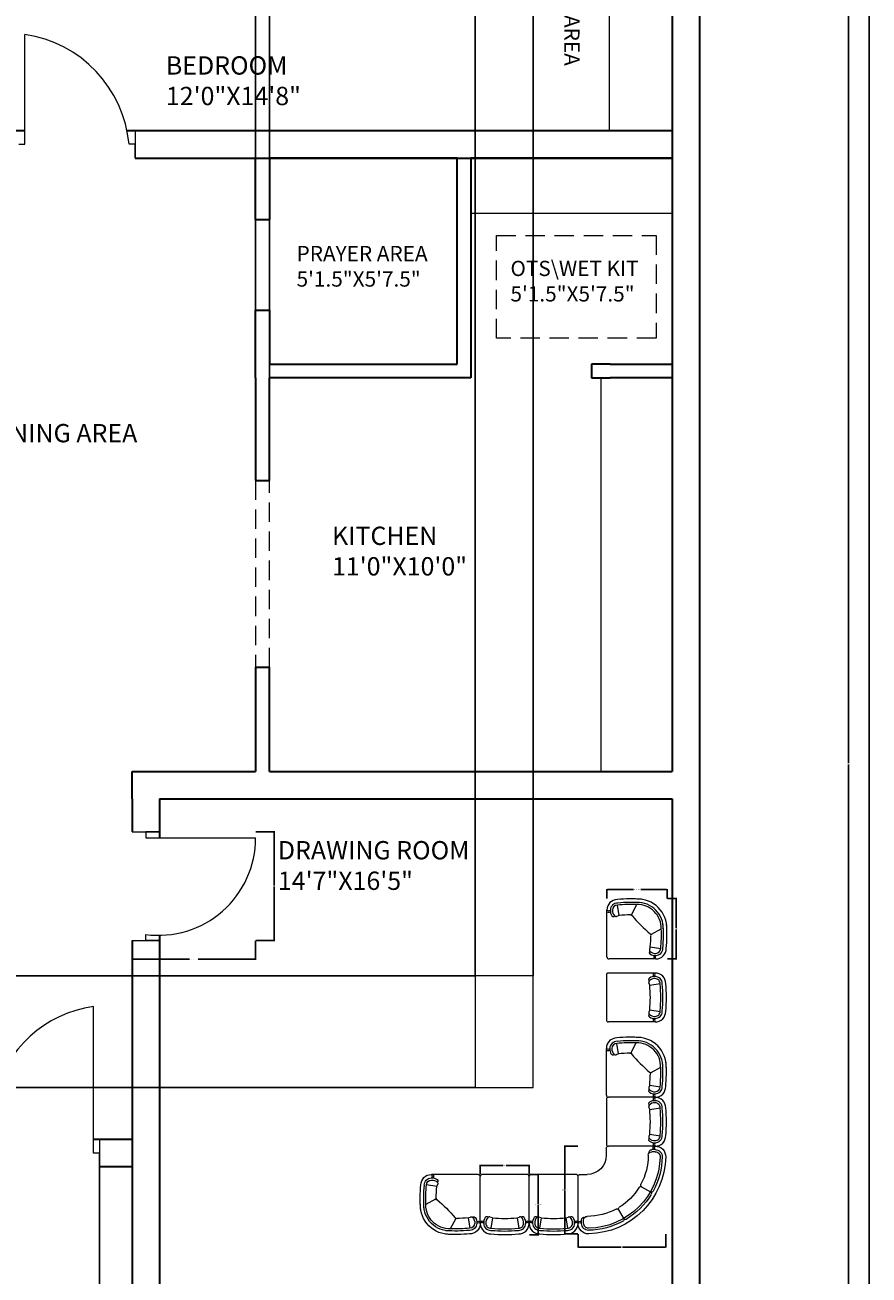
# Model space of a CAD drawing. Units: inches. Extents: x 2460 to 3031, y 933 to 2010.
# Tile 6 of 7: x 2754 to 3031, y 1339 to 1749. Entities that reach past the tile are written whole.
import ezdxf

# ---------------------------------------------------------------- set-up
doc = ezdxf.new("R2010")
doc.units = ezdxf.units.IN
doc.linetypes.add('DASHED2', pattern=[9.525, 6.35, -3.175])
for name, color, linetype, lineweight in [('A-ANNO-DIMS', 2, 'Continuous', 18), ('A-ANNO-TTLB', 7, 'Continuous', 25), ('A-AREA-IDEN', 7, 'Continuous', 18), ('A-DOOR', 4, 'Continuous', 18), ('A-FLOR-CASE', 9, 'Continuous', 18), ('A-FLOR-OVHD', 254, 'DASHED2', 13), ('A-FURN', 8, 'Continuous', 18), ('A-WALL', 7, 'Continuous', 35), ('A-WALL-OVHD', 254, 'DASHED2', 13), ('C-PROP', 7, 'Continuous', 35)]:
    doc.layers.add(name, color=color, linetype=linetype, lineweight=lineweight)
doc.styles.get("Standard").update_dxf_attribs({"font": 'arial.ttf'})
doc.dimstyles.get("Standard").update_dxf_attribs({"dimtxt": 0.18, "dimasz": 0.18, "dimexe": 0.18, "dimexo": 0.0625, "dimgap": 0.09, "dimtad": 0, "dimtih": 1, "dimtoh": 1, "dimdec": 4, "dimzin": 0, "dimdsep": 46, "dimtxsty": 'Standard', "dimcen": 0.09, "dimadec": 0, "dimazin": 0, "dimtfac": 1, "dimtdec": 4, "dimtofl": 0, "dimtmove": 0, "dimatfit": 3, "dimfxl": 1, "dimtolj": 1, "dimtzin": 0, "dimarcsym": 0})

# ---------------------------------------------------------------- blocks, each defined once
blk = doc.blocks.new('A$C707258B2')
at = {"color": 0}
for p, q in [((0.404, 0.342), (1.074, 0.342)), ((0.404, 0.292), (0.454, 0.292)), ((0.404, 0.262), (0.454, 0.262)), ((1.104, 0.312), (1.104, 0.212)), ((1.479, -0.063), (1.379, -0.063)), ((1.509, -0.763), (1.509, -0.093)), ((0.6, -0.238), (0.47, -0.313)), ((0.929, -0.567), (0.854, -0.697)), ((1.429, -0.763), (1.429, -0.713)), ((1.459, -0.763), (1.459, -0.712))]:
    blk.add_line(p, q, dxfattribs=at)
for centre, radius, start, end in [((0.404, 0.192), 0.15, 90, 181.1754), ((1.379, 0.212), 1.125, 181.1754, 268.8246), ((0.404, 0.192), 0.1, 90, 181.1754), ((1.379, 0.212), 1.075, 181.1754, 208.6357), ((0.404, 0.192), 0.07, 90, 181.1754), ((1.379, 0.212), 1.045, 181.1754, 268.8246), ((0.378, 0.317), 0.0362, 316.3972, 43.6028), ((0.368, 0.317), 0.0662, 337.8298, 22.1702), ((0.455, 0.256), 0.0357, 345.4262, 90.5555), ((0.454, 0.212), 0.05, 360, 90), ((1.379, 0.212), 0.875, 180, 208.4082), ((1.074, 0.312), 0.03, 360, 90), ((1.379, 0.212), 0.275, 180, 270), ((1.479, -0.093), 0.03, 360, 90), ((0.457, -0.291), 0.025, 208.6357, 300), ((0.482, -0.334), 0.025, 120, 211.3643), ((1.379, 0.212), 1.075, 211.3643, 238.6357), ((0.587, -0.216), 0.025, 300, 28.4082), ((0.612, -0.259), 0.025, 31.5918, 120), ((1.379, 0.212), 0.875, 211.5918, 238.4082), ((0.907, -0.555), 0.025, 330, 58.4082), ((0.832, -0.685), 0.025, 238.6357, 330), ((0.876, -0.71), 0.025, 150, 241.3643), ((0.951, -0.58), 0.025, 61.5918, 150), ((1.379, 0.212), 0.875, 241.5918, 270), ((1.379, -0.713), 0.05, 360, 90), ((1.425, -0.709), 0.0336, 354.6301, 109.3883), ((1.379, 0.212), 1.075, 241.3643, 268.8246), ((1.359, -0.763), 0.15, 268.8246, 360), ((1.359, -0.763), 0.1, 268.8246, 360), ((1.359, -0.763), 0.07, 268.8246, 360), ((1.484, -0.799), 0.0662, 67.8298, 112.1702), ((1.484, -0.789), 0.0362, 46.3972, 133.6028)]:
    blk.add_arc(centre, radius, start, end, dxfattribs=at)
blk = doc.blocks.new('part 01')
at = {"color": 0}
for p, q in [((-591, 527), (-740, 550)), ((-670, 700), (0, 700)), ((-591, 527), (-579, 561)), ((30, 30), (30, 670)), ((-591, 173), (-740, 150)), ((-670, 0), (0, 0)), ((-591, 173), (-579, 139))]:
    blk.add_line(p, q, dxfattribs=at)
for centre, radius, start, end in [((1178, 350), 2008, 174.2835, 185.7165), ((-670, 550), 150, 90, 181.1754), ((1178, 350), 1958, 174.2835, 185.7165), ((-670, 550), 100, 90, 181.1754), ((1178, 350), 1928, 174.2835, 185.7165), ((-670, 550), 70, 90, 181.1754), ((-660, 518), 133, 56.0897, 95.6132), ((-696, 675), 36.2, 316.3972, 43.6028), ((-660, 518), 103, 42.0066, 95.6132), ((-706, 675), 66.2, 337.8298, 22.1702), ((-600, 607), 25, 332.9608, 56.0897), ((-625, 620), 53.2, 321.0017, 332.9608), ((-602, 570), 25, 340, 42.0066), ((0, 670), 30, 0, 90), ((1178, 350), 1778, 174.2835, 185.7165), ((-670, 150), 150, 178.8246, 270), ((-670, 150), 100, 178.8246, 270), ((-670, 150), 70, 178.8246, 270), ((-660, 182), 133, 264.3868, 303.9103), ((-660, 182), 103, 264.3868, 317.9934), ((-696, 25), 36.2, 316.3972, 43.6028), ((-706, 25), 66.2, 337.8298, 22.1702), ((-600, 93), 25, 303.9103, 27.0392), ((-602, 130), 25, 317.9934, 20), ((-625, 80), 53.2, 27.0392, 38.9983), ((0, 30), 30, 270, 0)]:
    blk.add_arc(centre, radius, start, end, dxfattribs=at)
blk = doc.blocks.new('part02')
at = {"color": 0}
for p, q in [((0, -670), (0, 0)), ((30, 30), (700, 30)), ((621, -143), (609, -109)), ((621, -143), (770, -120)), ((640, -326), (778, -399)), ((173, -591), (139, -579)), ((173, -591), (150, -740)), ((356, -610), (429, -748))]:
    blk.add_line(p, q, dxfattribs=at)
for centre, radius, start, end in [((30, 0), 30, 90, 180), ((726, 5), 56.2, 153.6122, 206.6666), ((726, 5), 36.2, 136.3972, 223.6028), ((700, -120), 150, 0, 90), ((630, -63), 25, 123.9103, 207.0392), ((655, -50), 53.2, 207.0392, 218.9983), ((632, -100), 25, 137.9934, 200), ((690, -152), 103, 84.3868, 137.9934), ((689, -151), 132, 85.4378, 123.9887), ((-1148, -320), 1778, 0.3836, 5.7165), ((700, -121), 101, 357.5006, 89.858), ((700, -120), 70, 0, 90), ((-1228, -320), 2008, 357.7349, 5.7032), ((-1148, -320), 1958, 355.8657, 5.7165), ((-1148, -320), 2008, 355.818, 5.7165), ((2220, -2190), 2454, 130.6961, 139.3039), ((632, -344), 20, 62, 130.6961), ((650, -308), 20, 180.3836, 242), ((439, -409), 419, 268.2181, 1.7819), ((439, -409), 369, 268.2181, 1.7819), ((439, -409), 339, 268.2181, 1.7819), ((25, -696), 56.2, 63.3334, 116.3878), ((25, -696), 36.2, 46.3972, 133.6028), ((150, -670), 150, 180, 271.1754), ((182, -660), 133, 146.0897, 185.6132), ((150, -670), 100, 180, 271.1754), ((93, -600), 25, 62.9608, 146.0897), ((182, -660), 103, 132.0066, 185.6132), ((150, -670), 70, 180, 270), ((80, -625), 53.2, 51.0017, 62.9608), ((130, -602), 25, 70, 132.0066), ((350, 1178), 1778, 264.2835, 269.6164), ((338, -620), 20, 28, 89.6164), ((374, -602), 20, 139.3039, 208), ((350, 1258), 2008, 264.2968, 272.2651), ((350, 1178), 2008, 264.2835, 274.182), ((350, 1178), 1958, 264.2835, 274.1343)]:
    blk.add_arc(centre, radius, start, end, dxfattribs=at)
blk = doc.blocks.new('DOOR-SWING-36')
for p, q in [((0, 35.65), (9, 35.65)), ((4.5, 35.65), (4.5, 33.65)), ((4.5, 33.65), (40.5, 33.65)), ((4.5, 0), (4.5, 2)), ((0, 0), (9, 0)), ((9, 0), (4.5, 0))]:
    blk.add_line(p, q)
blk.add_arc((8.58, 33.65), 31.92, 262.6481, 0)
blk = doc.blocks.new('*D18')
at = {"layer": 'A-ANNO-DIMS', "color": 0, "lineweight": -2, "transparency": 16777216}
for p, q in [((2919.36, 1372.43), (2922.44, 1372.43)), ((2922.26, 1372.25), (2922.26, 1362.73)), ((2922.26, 1352.85), (2922.26, 1362.37)), ((2919.36, 1352.67), (2922.44, 1352.67))]:
    blk.add_line(p, q, dxfattribs=at)
at = {"layer": 'A-ANNO-DIMS', "color": 0, "transparency": 16777216}
for points in [[(2922.23, 1372.25), (2922.29, 1372.25), (2922.26, 1372.43)], [(2922.23, 1352.85), (2922.29, 1352.85), (2922.26, 1352.67)]]:
    blk.add_solid(points, dxfattribs=at)
at = {"layer": 'Defpoints', "color": 0, "transparency": 16777216}
for p in [(2919.29, 1372.43), (2922.26, 1372.43), (2919.29, 1352.67)]:
    blk.add_point(p, dxfattribs=at)
at = {"layer": 'A-ANNO-DIMS', "color": 0, "transparency": 16777216, "insert": (2922.26, 1362.55), "char_height": 0.18, "attachment_point": 5}
blk.add_mtext('\\A1;SOFA SEAT 20 TYP.', dxfattribs=at)
blk = doc.blocks.new('*D19')
at = {"layer": 'A-ANNO-DIMS', "color": 0, "lineweight": -2, "transparency": 16777216}
for p, q in [((2903.27, 1372.49), (2903.27, 1375.57)), ((2903.45, 1375.39), (2910.76, 1375.39)), ((2919.11, 1375.39), (2911.8, 1375.39)), ((2919.29, 1372.49), (2919.29, 1375.57))]:
    blk.add_line(p, q, dxfattribs=at)
at = {"layer": 'A-ANNO-DIMS', "color": 0, "transparency": 16777216}
for points in [[(2903.45, 1375.42), (2903.45, 1375.36), (2903.27, 1375.39)], [(2919.11, 1375.42), (2919.11, 1375.36), (2919.29, 1375.39)]]:
    blk.add_solid(points, dxfattribs=at)
at = {"layer": 'Defpoints', "color": 0, "transparency": 16777216}
for p in [(2903.27, 1375.39), (2903.27, 1372.43), (2919.29, 1372.43)]:
    blk.add_point(p, dxfattribs=at)
at = {"layer": 'A-ANNO-DIMS', "color": 0, "transparency": 16777216, "insert": (2911.28, 1375.39), "char_height": 0.18, "attachment_point": 5}
blk.add_mtext('\\A1;16 TYP.', dxfattribs=at)
blk = doc.blocks.new('*D20')
at = {"layer": 'A-ANNO-DIMS', "color": 0, "lineweight": -2, "transparency": 16777216}
for p, q in [((2944.78, 1462.86), (2944.78, 1465.94)), ((2944.96, 1465.76), (2953.47, 1465.76)), ((2964.35, 1465.76), (2955.84, 1465.76)), ((2964.53, 1462.86), (2964.53, 1465.94))]:
    blk.add_line(p, q, dxfattribs=at)
at = {"layer": 'A-ANNO-DIMS', "color": 0, "transparency": 16777216}
for points in [[(2944.96, 1465.79), (2944.96, 1465.73), (2944.78, 1465.76)], [(2964.35, 1465.79), (2964.35, 1465.73), (2964.53, 1465.76)]]:
    blk.add_solid(points, dxfattribs=at)
at = {"layer": 'Defpoints', "color": 0, "transparency": 16777216}
for p in [(2944.78, 1465.76), (2944.78, 1462.8), (2964.53, 1462.8)]:
    blk.add_point(p, dxfattribs=at)
at = {"layer": 'A-ANNO-DIMS', "color": 0, "transparency": 16777216, "insert": (2954.65, 1465.76), "char_height": 0.18, "attachment_point": 5}
blk.add_mtext('\\A1;END SEAT 20 TYP.', dxfattribs=at)
blk = doc.blocks.new('*D21')
at = {"layer": 'A-ANNO-DIMS', "color": 0, "lineweight": -2, "transparency": 16777216}
for p, q in [((2964.59, 1462.8), (2967.67, 1462.8)), ((2967.49, 1462.62), (2967.49, 1453.1)), ((2967.49, 1443.22), (2967.49, 1452.74)), ((2964.59, 1443.04), (2967.67, 1443.04))]:
    blk.add_line(p, q, dxfattribs=at)
at = {"layer": 'A-ANNO-DIMS', "color": 0, "transparency": 16777216}
for points in [[(2967.46, 1462.62), (2967.52, 1462.62), (2967.49, 1462.8)], [(2967.46, 1443.22), (2967.52, 1443.22), (2967.49, 1443.04)]]:
    blk.add_solid(points, dxfattribs=at)
at = {"layer": 'Defpoints', "color": 0, "transparency": 16777216}
for p in [(2964.53, 1462.8), (2967.49, 1462.8), (2964.53, 1443.04)]:
    blk.add_point(p, dxfattribs=at)
at = {"layer": 'A-ANNO-DIMS', "color": 0, "transparency": 16777216, "insert": (2967.49, 1452.92), "char_height": 0.18, "attachment_point": 5}
blk.add_mtext('\\A1;20 TYP.', dxfattribs=at)
blk = doc.blocks.new('*D22')
at = {"layer": 'A-ANNO-DIMS', "color": 0, "lineweight": -2, "transparency": 16777216}
for p, q in [((2935.25, 1381.7), (2930.82, 1381.7)), ((2931, 1381.52), (2931, 1367.51)), ((2931, 1353.14), (2931, 1367.14)), ((2935.25, 1352.96), (2930.82, 1352.96))]:
    blk.add_line(p, q, dxfattribs=at)
at = {"layer": 'A-ANNO-DIMS', "color": 0, "transparency": 16777216}
for points in [[(2930.97, 1381.52), (2931.03, 1381.52), (2931, 1381.7)], [(2930.97, 1353.14), (2931.03, 1353.14), (2931, 1352.96)]]:
    blk.add_solid(points, dxfattribs=at)
at = {"layer": 'Defpoints', "color": 0, "transparency": 16777216}
for p in [(2931, 1381.7), (2935.32, 1381.7), (2935.32, 1352.96)]:
    blk.add_point(p, dxfattribs=at)
at = {"layer": 'A-ANNO-DIMS', "color": 0, "transparency": 16777216, "insert": (2931, 1367.33), "char_height": 0.18, "attachment_point": 5}
blk.add_mtext('\\A1;CORNER SEAT 29', dxfattribs=at)
blk = doc.blocks.new('*D23')
at = {"layer": 'A-ANNO-DIMS', "color": 0, "lineweight": -2, "transparency": 16777216}
for p, q in [((2935.32, 1352.9), (2935.32, 1348.47)), ((2964.06, 1352.9), (2964.06, 1348.47)), ((2935.5, 1348.65), (2949.46, 1348.65)), ((2963.88, 1348.65), (2949.91, 1348.65))]:
    blk.add_line(p, q, dxfattribs=at)
at = {"layer": 'A-ANNO-DIMS', "color": 0, "transparency": 16777216}
for points in [[(2935.5, 1348.68), (2935.5, 1348.62), (2935.32, 1348.65)], [(2963.88, 1348.68), (2963.88, 1348.62), (2964.06, 1348.65)]]:
    blk.add_solid(points, dxfattribs=at)
at = {"layer": 'Defpoints', "color": 0, "transparency": 16777216}
for p in [(2935.32, 1352.96), (2964.06, 1352.96), (2935.32, 1348.65)]:
    blk.add_point(p, dxfattribs=at)
at = {"layer": 'A-ANNO-DIMS', "color": 0, "transparency": 16777216, "insert": (2949.69, 1348.65), "char_height": 0.18, "attachment_point": 5}
blk.add_mtext('\\A1;29', dxfattribs=at)
blk = doc.blocks.new('*D24')
at = {"layer": 'A-ANNO-DIMS', "color": 0, "lineweight": -2, "transparency": 16777216}
for p, q in [((2789.17, 1448.99), (2789.17, 1442.8)), ((2829.67, 1448.99), (2829.67, 1442.8)), ((2789.35, 1442.98), (2808.02, 1442.98)), ((2829.49, 1442.98), (2810.82, 1442.98))]:
    blk.add_line(p, q, dxfattribs=at)
at = {"layer": 'A-ANNO-DIMS', "color": 0, "transparency": 16777216}
for points in [[(2789.35, 1443.01), (2789.35, 1442.95), (2789.17, 1442.98)], [(2829.49, 1443.01), (2829.49, 1442.95), (2829.67, 1442.98)]]:
    blk.add_solid(points, dxfattribs=at)
at = {"layer": 'Defpoints', "color": 0, "transparency": 16777216}
for p in [(2789.17, 1449.05), (2829.67, 1449.05), (2829.67, 1442.98)]:
    blk.add_point(p, dxfattribs=at)
at = {"layer": 'A-ANNO-DIMS', "color": 0, "transparency": 16777216, "insert": (2809.42, 1442.98), "char_height": 0.18, "attachment_point": 5}
blk.add_mtext('\\A1;DOOR SWING 41 TYP.', dxfattribs=at)
blk = doc.blocks.new('*D25')
at = {"layer": 'A-ANNO-DIMS', "color": 0, "lineweight": -2, "transparency": 16777216}
for p, q in [((2829.73, 1484.71), (2835.92, 1484.71)), ((2835.74, 1484.53), (2835.74, 1467.06)), ((2835.74, 1449.23), (2835.74, 1466.7)), ((2829.73, 1449.05), (2835.92, 1449.05))]:
    blk.add_line(p, q, dxfattribs=at)
at = {"layer": 'A-ANNO-DIMS', "color": 0, "transparency": 16777216}
for points in [[(2835.71, 1484.53), (2835.77, 1484.53), (2835.74, 1484.71)], [(2835.71, 1449.23), (2835.77, 1449.23), (2835.74, 1449.05)]]:
    blk.add_solid(points, dxfattribs=at)
at = {"layer": 'Defpoints', "color": 0, "transparency": 16777216}
for p in [(2829.67, 1484.71), (2835.74, 1484.71), (2829.67, 1449.05)]:
    blk.add_point(p, dxfattribs=at)
at = {"layer": 'A-ANNO-DIMS', "color": 0, "transparency": 16777216, "insert": (2835.74, 1466.88), "char_height": 0.18, "attachment_point": 5}
blk.add_mtext('\\A1;36 TYP.', dxfattribs=at)
blk = doc.blocks.new('*D33')
at = {"layer": 'A-ANNO-DIMS', "color": 0, "lineweight": -2, "transparency": 16777216}
for p, q in [((2975.23, 1957.98), (3024.15, 1957.98)), ((3023.97, 1957.8), (3023.97, 1507.16)), ((3023.97, 1056.16), (3023.97, 1506.8)), ((2975.23, 1055.98), (3024.15, 1055.98))]:
    blk.add_line(p, q, dxfattribs=at)
at = {"layer": 'A-ANNO-DIMS', "color": 0, "transparency": 16777216}
for points in [[(3023.94, 1957.8), (3024, 1957.8), (3023.97, 1957.98)], [(3023.94, 1056.16), (3024, 1056.16), (3023.97, 1055.98)]]:
    blk.add_solid(points, dxfattribs=at)
at = {"layer": 'Defpoints', "color": 0, "transparency": 16777216}
for p in [(2975.17, 1957.98), (3023.97, 1957.98), (2975.17, 1055.98)]:
    blk.add_point(p, dxfattribs=at)
at = {"layer": 'A-ANNO-DIMS', "color": 0, "transparency": 16777216, "insert": (3023.97, 1506.98), "char_height": 0.18, "attachment_point": 5}
blk.add_mtext('\\A1;902', dxfattribs=at)
blk = doc.blocks.new('*D41')
at = {"layer": 'A-ANNO-DIMS', "color": 0, "lineweight": -2, "transparency": 16777216}
for p, q in [((2829.67, 1599.92), (2829.67, 2006.96)), ((2829.85, 2006.78), (2831.66, 2006.78)), ((2833.99, 2006.78), (2832.18, 2006.78)), ((2834.17, 1599.92), (2834.17, 2006.96))]:
    blk.add_line(p, q, dxfattribs=at)
at = {"layer": 'A-ANNO-DIMS', "color": 0, "transparency": 16777216}
for points in [[(2829.85, 2006.81), (2829.85, 2006.75), (2829.67, 2006.78)], [(2833.99, 2006.81), (2833.99, 2006.75), (2834.17, 2006.78)]]:
    blk.add_solid(points, dxfattribs=at)
at = {"layer": 'Defpoints', "color": 0, "transparency": 16777216}
for p in [(2834.17, 2006.78), (2829.67, 1599.86), (2834.17, 1599.86)]:
    blk.add_point(p, dxfattribs=at)
at = {"layer": 'A-ANNO-DIMS', "color": 0, "transparency": 16777216, "insert": (2831.92, 2006.78), "char_height": 0.18, "attachment_point": 5}
blk.add_mtext('\\A1;4.5', dxfattribs=at)
blk = doc.blocks.new('*D43')
at = {"layer": 'A-ANNO-DIMS', "color": 0, "lineweight": -2, "transparency": 16777216}
for p, q in [((2707.62, 1374.89), (2707.62, 933.16)), ((2778.55, 1374.89), (2778.55, 933.16)), ((2707.8, 933.34), (2742.69, 933.34)), ((2778.37, 933.34), (2743.48, 933.34))]:
    blk.add_line(p, q, dxfattribs=at)
at = {"layer": 'A-ANNO-DIMS', "color": 0, "transparency": 16777216}
for points in [[(2707.8, 933.37), (2707.8, 933.31), (2707.62, 933.34)], [(2778.37, 933.37), (2778.37, 933.31), (2778.55, 933.34)]]:
    blk.add_solid(points, dxfattribs=at)
at = {"layer": 'Defpoints', "color": 0, "transparency": 16777216}
for p in [(2707.62, 1374.95), (2778.55, 1374.95), (2778.55, 933.34)]:
    blk.add_point(p, dxfattribs=at)
at = {"layer": 'A-ANNO-DIMS', "color": 0, "transparency": 16777216, "insert": (2743.09, 933.34), "char_height": 0.18, "attachment_point": 5}
blk.add_mtext('\\A1;70.93', dxfattribs=at)
blk = doc.blocks.new('*D49')
at = {"layer": 'A-ANNO-DIMS', "color": 0, "lineweight": -2, "transparency": 16777216}
for p, q in [((2901.62, 1437.52), (2901.62, 2006.96)), ((2901.8, 2006.78), (2910.66, 2006.78)), ((2920.43, 2006.78), (2911.57, 2006.78)), ((2920.61, 1437.52), (2920.61, 2006.96))]:
    blk.add_line(p, q, dxfattribs=at)
at = {"layer": 'A-ANNO-DIMS', "color": 0, "transparency": 16777216}
for points in [[(2901.8, 2006.81), (2901.8, 2006.75), (2901.62, 2006.78)], [(2920.43, 2006.81), (2920.43, 2006.75), (2920.61, 2006.78)]]:
    blk.add_solid(points, dxfattribs=at)
at = {"layer": 'Defpoints', "color": 0, "transparency": 16777216}
for p in [(2920.61, 2006.78), (2901.62, 1437.46), (2920.61, 1437.46)]:
    blk.add_point(p, dxfattribs=at)
at = {"layer": 'A-ANNO-DIMS', "color": 0, "transparency": 16777216, "insert": (2911.11, 2006.78), "char_height": 0.18, "attachment_point": 5}
blk.add_mtext('\\A1;18.996', dxfattribs=at)
blk = doc.blocks.new('*D50')
at = {"layer": 'A-ANNO-DIMS', "color": 0, "lineweight": -2, "transparency": 16777216}
for p, q in [((2901.55, 1437.46), (2462.69, 1437.46)), ((2462.87, 1437.28), (2462.87, 1419.38)), ((2462.87, 1401.12), (2462.87, 1419.02)), ((2901.55, 1400.94), (2462.69, 1400.94))]:
    blk.add_line(p, q, dxfattribs=at)
at = {"layer": 'A-ANNO-DIMS', "color": 0, "transparency": 16777216}
for points in [[(2462.84, 1437.28), (2462.9, 1437.28), (2462.87, 1437.46)], [(2462.84, 1401.12), (2462.9, 1401.12), (2462.87, 1400.94)]]:
    blk.add_solid(points, dxfattribs=at)
at = {"layer": 'Defpoints', "color": 0, "transparency": 16777216}
for p in [(2462.87, 1437.46), (2901.62, 1437.46), (2901.62, 1400.94)]:
    blk.add_point(p, dxfattribs=at)
at = {"layer": 'A-ANNO-DIMS', "color": 0, "transparency": 16777216, "insert": (2462.87, 1419.2), "char_height": 0.18, "attachment_point": 5}
blk.add_mtext('\\A1;36.524', dxfattribs=at)

msp = doc.modelspace()

# ---------------------------------------------------------------- linework, layer by layer
at = {"layer": 'A-ANNO-TTLB'}
msp.add_lwpolyline([(2459.8083, 2009.7942), (3030.6598, 2009.7942), (3030.6598, 936.3732), (2459.8083, 936.3732)], close=True, dxfattribs=at)
at = {"layer": 'A-DOOR'}
for p, q in [((2754.0876, 1709.9828), (2754.0876, 1745.9828)), ((2790.1713, 1714.4828), (2790.1713, 1705.4828)), ((2752.0876, 1709.9828), (2754.0876, 1709.9828)), ((2790.1713, 1709.9828), (2788.1713, 1709.9828)), ((2790.1713, 1705.4828), (2790.1713, 1709.9828)), ((2798.1684, 1484.7065), (2793.6684, 1484.7065)), ((2776.5542, 1379.4491), (2776.5542, 1427.4491)), ((2778.5542, 1383.9491), (2778.5542, 1374.9491)), ((2778.5542, 1379.4491), (2776.5542, 1379.4491)), ((2778.5542, 1374.9491), (2778.5542, 1379.4491))]:
    msp.add_line(p, q, dxfattribs=at)
for centre, radius, start, end in [((2748.2483, 1706.3196), 40.0908, 5.242641, 81.624947), ((2781.8372, 1389.0544), 38.7565, 97.834609, 166.856265)]:
    msp.add_arc(centre, radius, start, end, dxfattribs=at)
at = {"layer": 'A-FLOR-CASE'}
for p, q in [((2945.476, 1801.9828), (2945.476, 1714.4828)), ((2900.1684, 1687.4172), (2900.1684, 1687.4172)), ((2900.1684, 1687.4172), (2966.1684, 1687.4172)), ((2942.7629, 1633.4828), (2942.7629, 1504.4828))]:
    msp.add_line(p, q, dxfattribs=at)
at = {"layer": 'A-FLOR-OVHD'}
msp.add_lwpolyline([(2908.587, 1680.1056), (2960.8903, 1680.1056), (2960.8903, 1646.4564), (2908.587, 1646.4564)], close=True, dxfattribs=at)
at = {"layer": 'A-FURN'}
msp.add_lwpolyline([(2920.6119, 1437.4597), (2901.6162, 1437.4597), (2901.6162, 1400.9352), (2920.6119, 1400.9352)], close=True, dxfattribs=at)
at = {"layer": 'A-WALL'}
for p, q in [((2966.1684, 1801.9828), (2966.1684, 1504.4828)), ((2745.6684, 1714.4828), (2754.0876, 1714.4828)), ((2787.4991, 1714.4828), (2889.6684, 1714.4828)), ((2889.6684, 1714.4828), (2894.1684, 1714.4828)), ((2894.1684, 1714.4828), (2966.1684, 1714.4828)), ((2790.1713, 1705.4828), (2895.6684, 1705.4828)), ((2829.6684, 1685.3831), (2829.6684, 1705.4828)), ((2895.6684, 1705.4828), (2834.1684, 1705.4828)), ((2834.1684, 1705.4828), (2834.1684, 1685.3831)), ((2894.1684, 1705.4828), (2966.1684, 1705.4828)), ((2895.6684, 1637.9828), (2895.6684, 1705.4828)), ((2966.1684, 1705.4828), (2900.1684, 1705.4828)), ((2900.1684, 1705.4828), (2900.1684, 1637.9828)), ((2829.6684, 1685.3831), (2834.1684, 1685.3831)), ((2829.6684, 1633.4828), (2829.6684, 1655.6634)), ((2829.6684, 1655.6634), (2834.1684, 1655.6634)), ((2834.1684, 1655.6634), (2834.1684, 1637.9828)), ((2834.1684, 1637.9828), (2895.6684, 1637.9828)), ((2900.1684, 1637.9828), (2900.1684, 1633.4828)), ((2945.8477, 1637.9828), (2939.6781, 1637.9828)), ((2939.6781, 1637.9828), (2939.6781, 1633.4828)), ((2945.8477, 1637.9828), (2966.1684, 1637.9828)), ((2966.1684, 1637.9828), (2966.1684, 1633.4828)), ((2829.6684, 1633.4828), (2829.6684, 1599.86)), ((2895.6684, 1633.4828), (2834.1684, 1633.4828)), ((2834.1684, 1599.86), (2834.1684, 1633.4828)), ((2900.1684, 1633.4828), (2895.6684, 1633.4828)), ((2939.6781, 1633.4828), (2945.8477, 1633.4828)), ((2966.1684, 1633.4828), (2945.8477, 1633.4828)), ((2829.6684, 1599.86), (2834.1684, 1599.86)), ((2829.6684, 1538.6366), (2834.1684, 1538.6366)), ((2829.6684, 1538.6366), (2829.6684, 1504.4828)), ((2834.1684, 1504.4828), (2834.1684, 1538.6366)), ((2789.1684, 1495.4828), (2789.1684, 1504.4828)), ((2789.1684, 1504.4828), (2829.6684, 1504.4828)), ((2834.1684, 1504.4828), (2966.1684, 1504.4828)), ((2894.1684, 1504.4828), (2966.1684, 1504.4828)), ((2789.1684, 1495.4828), (2789.1684, 1484.7065)), ((2798.1684, 1495.4828), (2798.1684, 1482.7065)), ((2798.1684, 1495.4828), (2966.1684, 1495.4828)), ((2894.1684, 1495.4828), (2966.1684, 1495.4828)), ((2966.1684, 1495.4828), (2966.1684, 1295.9828)), ((2798.1684, 1450.7932), (2798.1684, 1295.9828)), ((2789.1684, 1449.0529), (2789.1684, 1286.9828)), ((2776.5542, 1383.9491), (2789.1684, 1383.9491)), ((2789.1684, 1383.9491), (2789.1684, 1374.9491)), ((2789.1684, 1374.9491), (2778.5542, 1374.9491))]:
    msp.add_line(p, q, dxfattribs=at)
at = {"layer": 'A-WALL-OVHD'}
for p, q in [((2829.6684, 1685.3831), (2829.6684, 1655.6634)), ((2834.1684, 1685.3831), (2834.1684, 1655.6634)), ((2829.6684, 1655.6634), (2829.6684, 1655.6634)), ((2829.6684, 1599.86), (2829.6684, 1538.6366)), ((2834.1684, 1538.6366), (2834.1684, 1599.86))]:
    msp.add_line(p, q, dxfattribs=at)
at = {"layer": 'C-PROP'}
msp.add_line((2975.1684, 1957.9828), (2975.1684, 1055.9828), dxfattribs=at)

# ---------------------------------------------------------------- block references
at = {"layer": 'A-DOOR'}
msp.add_blockref('DOOR-SWING-36', (2789.168, 1449.053), dxfattribs=at)
at = {"layer": 'A-FURN', "ltscale": 0.03}
for name, p, xscale, yscale, zscale, rotation in [('part02', (2945.4646, 1443.0445), 0.0228894426027535, 0.0228894426027535, 0.0228894426027535, 90), ('part 01', (2945.2726, 1438.4253), 0.0228894426027535, 0.0228894426027535, 0.0228894426027535, 180), ('part02', (2945.2726, 1397.7202), 0.0228894426027535, 0.0228894426027535, 0.0228894426027535, 90), ('part 01', (2945.2726, 1397.7202), 0.0228894426027535, 0.0228894426027535, 0.0228894426027535, 180), ('A$C707258B2', (2969.8547, 1373.8689), -22.88944260275347, 22.88944260275347, 22.88944260275347, 359.9999999999968), ('part02', (2903.2705, 1371.7407), -0.0228894426027535, 0.0228894426027535, 0.0228894426027535, 359.9999999999968), ('part 01', (2919.2931, 1371.7407), 0.0228894426027535, 0.0228894426027535, 0.0228894426027535, 90), ('part 01', (2935.3157, 1371.7407), 0.0228894426027535, 0.0228894426027535, 0.0228894426027535, 90)]:
    msp.add_blockref(name, p, dxfattribs=dict(at, xscale=xscale, yscale=yscale, zscale=zscale, rotation=rotation))

# ---------------------------------------------------------------- texts
at = {"layer": 'A-AREA-IDEN', "insert": (2935.8013, 1786.6763), "char_height": 5, "attachment_point": 1, "rotation": 270}
msp.add_mtext_dynamic_manual_height_columns('DRESSING AREA\\P6\'X8\'6"', width=124.82599, gutter_width=12.5, heights=[0], dxfattribs=at)
at = {"layer": 'A-AREA-IDEN', "attachment_point": 1}
for s, width, insert, char_height in [('BEDROOM\\P12\'0"X14\'8"', 93.706153, (2800.2575, 1738.8207), 6), ('PRAYER AREA\\P5\'1.5"X5\'7.5"', 92.093383, (2843.0808, 1676.6838), 5), ('OTS\\\\WET KIT\\P5\'1.5"X5\'7.5"', 92.093383, (2913.162, 1671.814), 5), ('LOBBY\\\\DINING AREA\\P20\'0"16\'9"', 152.675752, (2712.3561, 1618.3354), 6), ('KITCHEN\\P11\'0"X10\'0"', 111.477233, (2854.6912, 1584.6986), 6), ('DRAWING ROOM\\P14\'7"X16\'5"', 79.110619, (2836.9528, 1481.6714), 6)]:
    msp.add_mtext_dynamic_manual_height_columns(s, width=width, gutter_width=12.5, heights=[0], dxfattribs=dict(at, insert=insert, char_height=char_height))

# ---------------------------------------------------------------- dimensions: what is measured, and where the dimension line sits
at = {"layer": 'A-ANNO-DIMS'}
for base, p1, p2, override, picture, middle in [((2834.1684, 2006.7823), (2829.6684, 1599.86), (2834.1684, 1599.86), {"dimdec": 1, "dimlfac": 1, "dimrnd": 0, "dimzin": 0, "dimdsep": 46, "dimlunit": 2}, '*D41', (2831.9184, 2006.7823)), ((2920.6119, 2006.7823), (2901.6162, 1437.4597), (2920.6119, 1437.4597), {"dimdec": 3, "dimlfac": 1, "dimrnd": 0, "dimzin": 0, "dimdsep": 46, "dimlunit": 2}, '*D49', (2911.1141, 2006.7823)), ((2778.5542, 933.3411), (2707.6216, 1374.9491), (2778.5542, 1374.9491), {"dimdec": 2, "dimlfac": 1, "dimrnd": 0, "dimzin": 0, "dimdsep": 46, "dimlunit": 2}, '*D43', (2743.0879, 933.3411))]:
    dim = msp.add_linear_dim(base=base, p1=p1, p2=p2, dimstyle='Standard', override=override, dxfattribs=at)
    dim.commit()
    dim.dimension.update_dxf_attribs({"geometry": picture, "text_midpoint": middle})
for base, p1, p2, angle, override, picture, middle in [((3023.9679, 1957.9828), (2975.1684, 1055.9828), (2975.1684, 1957.9828), 90, {"dimdec": 0, "dimlfac": 1, "dimrnd": 0, "dimzin": 0, "dimdsep": 46, "dimlunit": 2}, '*D33', (3023.9679, 1506.9828)), ((2462.86893, 1437.45968), (2901.61619, 1400.93524), (2901.61619, 1437.45968), 90, {"dimdec": 3, "dimlfac": 1, "dimrnd": 0, "dimzin": 0, "dimdsep": 46, "dimlunit": 2}, '*D50', (2462.86893, 1419.19746)), ((2935.3157, 1348.6468), (2964.0555, 1352.9578), (2935.3157, 1352.9578), 180, {"dimdec": 0, "dimlfac": 1, "dimrnd": 0, "dimzin": 0, "dimdsep": 46, "dimlunit": 2}, '*D23', (2949.6856, 1348.6468))]:
    dim = msp.add_linear_dim(base=base, p1=p1, p2=p2, angle=angle, dimstyle='Standard', override=override, dxfattribs=at)
    dim.commit()
    dim.dimension.update_dxf_attribs({"geometry": picture, "text_midpoint": middle})
for base, p1, p2, angle, text, picture, middle in [((2835.7434, 1484.7065), (2829.6684, 1449.0529), (2829.6684, 1484.7065), 90, '<> TYP.', '*D25', (2835.7434, 1466.8797)), ((2944.7779, 1465.7577), (2964.5285, 1462.7951), (2944.7779, 1462.7951), 180, 'END SEAT <> TYP.', '*D20', (2954.6532, 1465.7577)), ((2967.4911, 1462.7951), (2964.5285, 1443.0445), (2964.5285, 1462.7951), 90, '<> TYP.', '*D21', (2967.4911, 1452.9198)), ((2931.0048, 1381.6976), (2935.3157, 1352.9578), (2935.3157, 1381.6976), 90, 'CORNER SEAT <>', '*D22', (2931.0048, 1367.3277)), ((2903.2705, 1375.3908), (2919.2931, 1372.4273), (2903.2705, 1372.4273), 180, '<> TYP.', '*D19', (2911.2818, 1375.3908)), ((2922.2565, 1372.4273), (2919.2931, 1352.6713), (2919.2931, 1372.4273), 90, 'SOFA SEAT <> TYP.', '*D18', (2922.2565, 1362.5493))]:
    dim = msp.add_linear_dim(base=base, p1=p1, p2=p2, angle=angle, text=text, dimstyle='Standard', override={"dimdec": 0, "dimlfac": 1, "dimrnd": 0, "dimzin": 0, "dimdsep": 46, "dimlunit": 2}, dxfattribs=at)
    dim.commit()
    dim.dimension.update_dxf_attribs({"geometry": picture, "text_midpoint": middle})
dim = msp.add_linear_dim(base=(2829.6684287001, 1442.9778782446), p1=(2789.1684287001, 1449.0528782446), p2=(2829.6684287001, 1449.0528782446), text='DOOR SWING <> TYP.', dimstyle='Standard', override={"dimdec": 0, "dimlfac": 1, "dimrnd": 0, "dimzin": 0, "dimdsep": 46, "dimlunit": 2}, dxfattribs=at)
dim.commit()
dim.dimension.update_dxf_attribs({"geometry": '*D24', "text_midpoint": (2809.4184287001, 1442.9778782446)})

doc.saveas('drawing.dxf')
